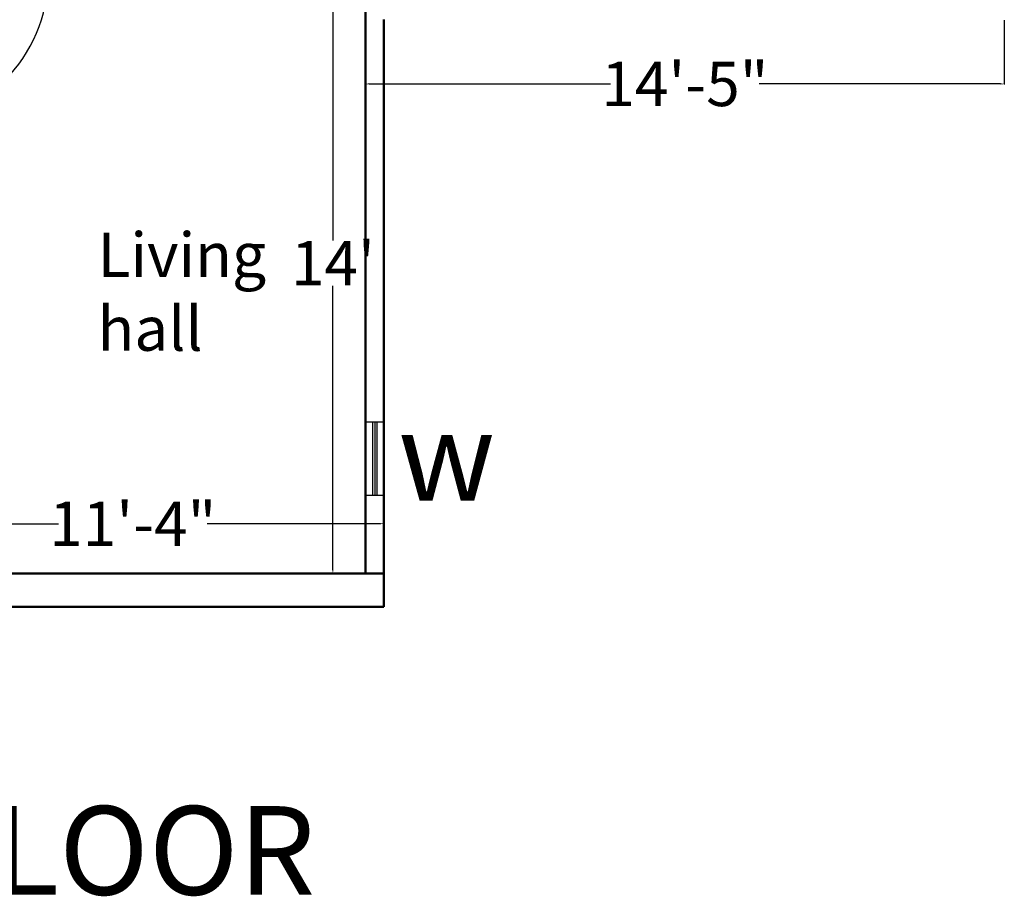
# Model space of a CAD drawing. Units: inches. Extents: x 409 to 7572, y 7 to 725.
# Tile 31 of 38: x 5952 to 6219, y 78 to 315. Entities that reach past the tile are written whole.
import ezdxf

# ---------------------------------------------------------------- set-up
doc = ezdxf.new("R2010")
doc.units = ezdxf.units.IN
doc.header["$MEASUREMENT"] = 0
for name, color, linetype, lineweight in [('A-ANNO-DIMS', 2, 'Continuous', 18), ('A-ANNO-SYMB', 3, 'Continuous', 25), ('A-ANNO-TEXT', 7, 'Continuous', 35), ('A-AREA-IDEN', 7, 'Continuous', 25), ('A-DOOR', 3, 'Continuous', 25), ('A-GLAZ', 4, 'Continuous', 25), ('A-WALL', 7, 'Continuous', 50)]:
    doc.layers.add(name, color=color, linetype=linetype, lineweight=lineweight)
doc.styles.get("Standard").update_dxf_attribs({"font": 'arial.ttf'})
doc.dimstyles.get("Standard").update_dxf_attribs({"dimtxt": 2, "dimasz": 1, "dimexe": 0.18, "dimexo": 0.0625, "dimgap": 0.09, "dimtad": 0, "dimtih": 1, "dimtoh": 1, "dimdec": 0, "dimzin": 0, "dimdsep": 46, "dimlunit": 3, "dimtxsty": 'Standard', "dimcen": 0.09, "dimadec": 0, "dimazin": 0, "dimtfac": 1, "dimtdec": 0, "dimtofl": 0, "dimtmove": 0, "dimatfit": 3, "dimfxl": 1, "dimtolj": 1, "dimtzin": 0, "dimarcsym": 0})

# ---------------------------------------------------------------- blocks, each defined once
blk = doc.blocks.new('*U5')
for p, q in [((0, 0), (0, 6)), ((40, 0), (40, 6))]:
    blk.add_line(p, q)
blk.add_lwpolyline([(0, 0), (0, -40), (1.75, -40), (1.75, 0)], close=True)
blk.add_arc((0, 0), 40, 270, 0)
blk = doc.blocks.new('*D123')
at = {"layer": 'A-ANNO-DIMS', "color": 0, "lineweight": -2, "transparency": 16777216}
for p, q in [((6045.72, 333.53), (6036.79, 333.53)), ((6036.97, 332.53), (6036.97, 255.65)), ((6036.97, 166.53), (6036.97, 243.42)), ((6045.72, 165.53), (6036.79, 165.53))]:
    blk.add_line(p, q, dxfattribs=at)
at = {"layer": 'A-ANNO-DIMS', "color": 0, "transparency": 16777216}
for points in [[(6036.8, 332.53), (6037.14, 332.53), (6036.97, 333.53)], [(6036.8, 166.53), (6037.14, 166.53), (6036.97, 165.53)]]:
    blk.add_solid(points, dxfattribs=at)
at = {"layer": 'DEFPOINTS', "color": 0, "transparency": 16777216}
for p in [(6045.78, 333.53), (6036.97, 165.53), (6045.78, 165.53)]:
    blk.add_point(p, dxfattribs=at)
at = {"layer": 'A-ANNO-DIMS', "color": 0, "transparency": 16777216, "insert": (6036.97, 249.53), "char_height": 2, "attachment_point": 5}
blk.add_mtext("\\A1;{\\H6x;14'}", dxfattribs=at)
blk = doc.blocks.new('*D124')
at = {"layer": 'A-ANNO-DIMS', "color": 0, "lineweight": -2, "transparency": 16777216}
for p, q in [((5914.78, 165.59), (5914.78, 179.18)), ((5915.78, 179), (5962.65, 179)), ((6049.78, 179), (6002.92, 179)), ((6050.78, 165.59), (6050.78, 179.18))]:
    blk.add_line(p, q, dxfattribs=at)
at = {"layer": 'A-ANNO-DIMS', "color": 0, "transparency": 16777216}
for points in [[(5915.78, 179.16), (5915.78, 178.83), (5914.78, 179)], [(6049.78, 179.16), (6049.78, 178.83), (6050.78, 179)]]:
    blk.add_solid(points, dxfattribs=at)
at = {"layer": 'DEFPOINTS', "color": 0, "transparency": 16777216}
for p in [(6050.78, 179), (5914.78, 165.53), (6050.78, 165.53)]:
    blk.add_point(p, dxfattribs=at)
at = {"layer": 'A-ANNO-DIMS', "color": 0, "transparency": 16777216, "insert": (5982.78, 179), "char_height": 2, "attachment_point": 5}
blk.add_mtext('\\A1;{\\H6x;11\'-4"}', dxfattribs=at)
blk = doc.blocks.new('*D147')
at = {"layer": 'A-ANNO-DIMS', "color": 0, "lineweight": -2, "transparency": 16777216}
for p, q in [((6045.78, 315.37), (6045.78, 297.9)), ((6218.78, 315.37), (6218.78, 297.9)), ((6046.78, 298.08), (6112.15, 298.08)), ((6217.78, 298.08), (6152.42, 298.08))]:
    blk.add_line(p, q, dxfattribs=at)
at = {"layer": 'A-ANNO-DIMS', "color": 0, "transparency": 16777216}
for points in [[(6046.78, 298.25), (6046.78, 297.92), (6045.78, 298.08)], [(6217.78, 298.25), (6217.78, 297.92), (6218.78, 298.08)]]:
    blk.add_solid(points, dxfattribs=at)
at = {"layer": 'DEFPOINTS', "color": 0, "transparency": 16777216}
for p in [(6045.78, 315.43), (6218.78, 315.43), (6218.78, 298.08)]:
    blk.add_point(p, dxfattribs=at)
at = {"layer": 'A-ANNO-DIMS', "color": 0, "transparency": 16777216, "insert": (6132.28, 298.08), "char_height": 2, "attachment_point": 5}
blk.add_mtext('\\A1;{\\H6x;14\'-5"}', dxfattribs=at)
blk = doc.blocks.new('WIN-20')
for p, q in [((2103.48, 182.68), (2083.54, 182.68)), ((2103.48, 182.13), (2083.54, 182.13)), ((2103.48, 181.57), (2083.54, 181.57))]:
    blk.add_line(p, q)
blk.add_lwpolyline([(2103.48, 179.64), (2083.54, 179.64), (2083.54, 184.62), (2103.48, 184.62)], close=True)

msp = doc.modelspace()

# ---------------------------------------------------------------- linework, layer by layer
at = {"layer": 'A-WALL'}
for p, q in [((6045.78, 333.53), (6045.78, 165.53)), ((6045.78, 333.53), (6045.78, 165.53)), ((6050.78, 315.53), (6050.78, 165.53)), ((5914.78, 165.53), (6050.78, 165.53)), ((6050.78, 165.53), (6050.78, 156.53)), ((5676.78, 156.53), (6050.78, 156.53))]:
    msp.add_line(p, q, dxfattribs=at)

# ---------------------------------------------------------------- block references
at = {"layer": 'A-DOOR'}
msp.add_blockref('*U5', (5919.84, 327.37), dxfattribs=at)
at = {"layer": 'A-GLAZ', "rotation": 89.99999999999905}
msp.add_blockref('WIN-20', (6230.42, -1896.94), dxfattribs=at)

# ---------------------------------------------------------------- texts
at = {"layer": 'A-ANNO-SYMB', "insert": (6054.64, 209.2), "char_height": 24, "attachment_point": 1}
msp.add_mtext_dynamic_manual_height_columns('w', width=18.2582, gutter_width=1, heights=[0], dxfattribs=at)
at = {"layer": 'A-ANNO-TEXT', "insert": (5789.44, 102.52), "char_height": 24, "attachment_point": 1}
msp.add_mtext_dynamic_manual_height_columns('FOURTH FLOOR', width=577.2242, gutter_width=1, heights=[0], dxfattribs=at)
at = {"layer": 'A-AREA-IDEN', "insert": (5973.25, 257.83), "char_height": 12, "attachment_point": 1}
msp.add_mtext_dynamic_manual_height_columns('Living hall', width=58.8843, gutter_width=1, heights=[0], dxfattribs=at)

# ---------------------------------------------------------------- dimensions: what is measured, and where the dimension line sits
at = {"layer": 'A-ANNO-DIMS'}
dim = msp.add_linear_dim(base=(6036.97, 165.53), p1=(6045.78, 333.53), p2=(6045.78, 165.53), angle=90, text='{\\H6x;<>}', dimstyle='Standard', override={"dimclrd": 0, "dimclre": 0, "dimclrt": 0}, dxfattribs=at)
dim.commit()
dim.dimension.update_dxf_attribs({"geometry": '*D123', "text_midpoint": (6036.97, 249.53)})
for base, p1, p2, picture, middle in [((6218.78, 298.08), (6045.78, 315.43), (6218.78, 315.43), '*D147', (6132.28, 298.08)), ((6050.78, 179), (5914.78, 165.53), (6050.78, 165.53), '*D124', (5982.78, 179))]:
    dim = msp.add_linear_dim(base=base, p1=p1, p2=p2, text='{\\H6x;<>}', dimstyle='Standard', override={"dimclrd": 0, "dimclre": 0, "dimclrt": 0}, dxfattribs=at)
    dim.commit()
    dim.dimension.update_dxf_attribs({"geometry": picture, "text_midpoint": middle})

doc.saveas('drawing.dxf')
